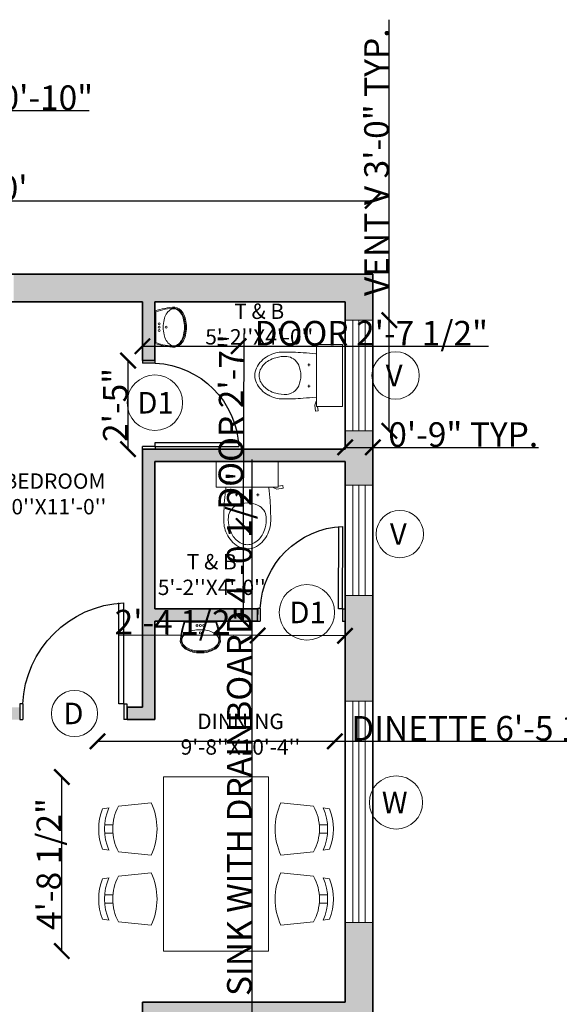
# Model space of a CAD drawing. Units: inches. Extents: x 2209 to 2954, y 1760 to 2265.
# Tile 4 of 7: x 2404 to 2580, y 1945 to 2265. Entities that reach past the tile are written whole.
import ezdxf

# ---------------------------------------------------------------- set-up
doc = ezdxf.new("R2010")
doc.units = ezdxf.units.IN
for name, color, linetype, lineweight in [('A-ANNO-DIMS', 2, 'Continuous', 18), ('A-ANNO-SYMB', 7, 'Continuous', 18), ('A-AREA-IDEN', 7, 'Continuous', 18), ('A-FLOR-FIXT', 9, 'Continuous', 18), ('A-FURN', 8, 'Continuous', 18), ('A-WALL-PATT', 30, 'Continuous', 13), ('DOOR', 240, 'Continuous', 25), ('WALL', 7, 'Continuous', 35), ('WINDOW', 190, 'Continuous', 18)]:
    doc.layers.add(name, color=color, linetype=linetype, lineweight=lineweight)
doc.styles.get("Standard").update_dxf_attribs({"font": 'arial.ttf'})
doc.dimstyles.get("Standard").update_dxf_attribs({"dimtxt": 8, "dimasz": 5, "dimexe": 0.18, "dimexo": 0.0625, "dimgap": 0.09, "dimtad": 1, "dimdec": 1, "dimzin": 0, "dimdsep": 46, "dimlunit": 4, "dimtxsty": 'Standard', "dimblk": 'ARCHTICK', "dimcen": 0.09, "dimse1": 1, "dimse2": 1, "dimadec": 0, "dimazin": 0, "dimtfac": 1, "dimtdec": 1, "dimtofl": 0, "dimtmove": 0, "dimatfit": 3, "dimfxl": 1, "dimtolj": 1, "dimtzin": 0, "dimarcsym": 0})

# ---------------------------------------------------------------- blocks, each defined once
blk = doc.blocks.new('table-23')
at = {"color": 0, "linetype": 'ByBlock'}
for p, q in [((-0.9, -1.4923), (-0.9, 0)), ((-0.9, 0), (0, 0)), ((0, -1.4923), (0, 0)), ((-1.0062, -0.2211), (-1.2862, -0.2511)), ((0.1062, -0.2211), (0.3862, -0.2511)), ((-1.3677, -0.2639), (-1.4237, -0.2726)), ((0.4677, -0.2639), (0.5237, -0.2726)), ((-1.4049, -0.4111), (-1.3347, -0.4111)), ((0.5049, -0.4111), (0.4347, -0.4111)), ((-1.4049, -0.4811), (-1.3347, -0.4811)), ((0.5049, -0.4811), (0.4347, -0.4811)), ((-1.3677, -0.6284), (-1.4237, -0.6197)), ((-1.0062, -0.6711), (-1.2862, -0.6411)), ((0.1062, -0.6711), (0.3862, -0.6411)), ((0.4677, -0.6284), (0.5237, -0.6197)), ((-1.0062, -0.8211), (-1.2862, -0.8511)), ((0.1062, -0.8211), (0.3862, -0.8511)), ((-1.3677, -0.8639), (-1.4237, -0.8726)), ((0.4677, -0.8639), (0.5237, -0.8726)), ((-1.4049, -1.0111), (-1.3347, -1.0111)), ((0.5049, -1.0111), (0.4347, -1.0111)), ((-1.4049, -1.0811), (-1.3347, -1.0811)), ((0.5049, -1.0811), (0.4347, -1.0811)), ((-1.3677, -1.2284), (-1.4237, -1.2197)), ((-1.0062, -1.2711), (-1.2862, -1.2411)), ((0.1062, -1.2711), (0.3862, -1.2411)), ((0.4677, -1.2284), (0.5237, -1.2197)), ((-0.9, -1.4923), (0, -1.4923))]:
    blk.add_line(p, q, dxfattribs=at)
for centre, radius, start, end in [((-0.931, -0.4461), 0.4053, 151.23721, 208.76279), ((-1.4875, -0.4461), 0.5312, 334.94238, 25.05762), ((0.5875, -0.4461), 0.5312, 154.94238, 205.05762), ((0.031, -0.4461), 0.4053, 331.23721, 28.76279), ((-0.9765, -0.4461), 0.4797, 158.78869, 201.21131), ((-0.9558, -0.4461), 0.4505, 156.13443, 203.86557), ((0.0558, -0.4461), 0.4505, 336.13443, 23.86557), ((0.0765, -0.4461), 0.4797, 338.78869, 21.21131), ((-1.4875, -1.0461), 0.5312, 334.94238, 25.05762), ((0.5875, -1.0461), 0.5312, 154.94238, 205.05762), ((-0.9765, -1.0461), 0.4797, 158.78869, 201.21131), ((-0.9558, -1.0461), 0.4505, 156.13443, 203.86557), ((-0.931, -1.0461), 0.4053, 151.23721, 208.76279), ((0.031, -1.0461), 0.4053, 331.23721, 28.76279), ((0.0558, -1.0461), 0.4505, 336.13443, 23.86557), ((0.0765, -1.0461), 0.4797, 338.78869, 21.21131)]:
    blk.add_arc(centre, radius, start, end, dxfattribs=at)
blk = doc.blocks.new('AP0B05')
for p, q in [((35, 100), (35, 880)), ((75, 100), (75, 878.9)), ((35, 100), (11, 100)), ((11, 100), (11, -20)), ((35, 100), (35, -20)), ((815, 100), (815, -20)), ((815, 100), (839, 100)), ((839, 100), (839, -20)), ((11, -20), (35, -20)), ((839, -20), (815, -20))]:
    blk.add_line(p, q)
blk.add_lwpolyline([(35, 100), (75, 100)])
blk.add_arc((-2.4, 62.6), 818.3, 2.62122, 87.37878)
blk = doc.blocks.new('toilet-1')
at = {"color": 0, "linetype": 'ByBlock'}
for p, q in [((-0.23, -0.02), (-0.23, -0.2116)), ((0.23, -0.02), (-0.23, -0.02)), ((0.23, -0.02), (0.23, -0.2116)), ((-0.23, -0.2116), (0.23, -0.2116)), ((0.1917, -0.2144), (0.2206, -0.225)), ((0.2206, -0.225), (0.266, -0.2187)), ((0.2633, -0.1997), (0.23, -0.2044)), ((0.266, -0.2187), (0.2633, -0.1997)), ((-0.0889, -0.2683), (-0.0697, -0.2683)), ((-0.0793, -0.2587), (-0.0793, -0.2778)), ((0.0889, -0.2683), (0.0698, -0.2683)), ((0.0794, -0.2587), (0.0794, -0.2778)), ((0, -0.6382), (0, -0.6382))]:
    blk.add_line(p, q, dxfattribs=at)
for centre, radius, start, end in [((3.5272, -0.6239), 3.7093, 173.69251, 175.15926), ((-3.527, -0.624), 3.7093, 4.84131, 6.31706), ((1.7368, -0.4519), 1.9109, 175.76982, 180.37578), ((-0.0312, -0.4465), 0.1114, 113.89968, 145.1485), ((0, -0.5169), 0.1884, 66.09393, 113.90607), ((0.0312, -0.4465), 0.1114, 34.8515, 66.10032), ((-1.7366, -0.4519), 1.9109, 359.62422, 4.23018), ((0.0981, -0.4497), 0.2389, 175.88621, 195.59308), ((-0.0408, -0.4398), 0.0996, 145.14967, 175.88096), ((0.0409, -0.4398), 0.0996, 4.11904, 34.85033), ((-0.098, -0.4497), 0.2389, 344.40692, 4.11379), ((0.0353, -0.463), 0.2093, 180.37466, 194.33753), ((-0.0351, -0.463), 0.2093, 345.6614, 359.62427), ((0.055, -0.458), 0.2297, 194.33532, 209.62204), ((0.0647, -0.4524), 0.2409, 209.62726, 224.54888), ((0.0961, -0.4503), 0.2369, 195.59686, 209.37705), ((0.0232, -0.4913), 0.1532, 209.38715, 226.54376), ((-0.0231, -0.4913), 0.1532, 313.45624, 330.61285), ((-0.0645, -0.4524), 0.2409, 315.45042, 330.37204), ((-0.096, -0.4503), 0.2369, 330.62295, 344.40314), ((-0.0548, -0.458), 0.2297, 330.37879, 345.66551), ((0.0178, -0.4986), 0.1751, 224.55199, 245.714), ((0.0152, -0.4997), 0.1416, 226.55015, 246.55272), ((0, -0.5347), 0.1034, 246.54933, 270.0042), ((0, -0.5347), 0.1034, 269.9958, 293.45067), ((-0.0151, -0.4997), 0.1416, 293.44728, 313.44985), ((-0.0176, -0.4986), 0.1751, 294.28649, 315.4485), ((0.0004, -0.538), 0.132, 245.58449, 269.87817), ((-0.0002, -0.538), 0.132, 270.12162, 294.4153)]:
    blk.add_arc(centre, radius, start, end, dxfattribs=at)
blk = doc.blocks.new('wash-3')
at = {"color": 0, "linetype": 'ByBlock'}
blk.add_line((0.23, -0.015), (-0.23, -0.015), dxfattribs=at)
for centre in [(-0.05, -0.066), (0, -0.066), (0.05, -0.066), (0, -0.172)]:
    blk.add_circle(centre, 0.0148, dxfattribs=at)
for centre, radius, start, end in [((0.69, -0.34), 0.991, 159.941, 177.839), ((0.69, -0.34), 0.976, 160.5399, 177.7326), ((-0.038, -0.45), 0.319, 103.3619, 119.8322), ((0, -0.61), 0.483, 90, 103.3619), ((0, -0.61), 0.483, 76.6381, 90), ((0.038, -0.45), 0.319, 60.1678, 76.6381), ((-0.69, -0.34), 0.976, 2.2674, 19.4601), ((-0.69, -0.34), 0.991, 2.161, 20.059), ((-0.183, -0.286), 0.095, 144.1588, 180), ((-0.183, -0.286), 0.095, 180, 215.8412), ((-0.096, -0.349), 0.203, 119.8322, 144.1588), ((0.096, -0.349), 0.203, 35.8412, 60.1678), ((0.183, -0.286), 0.095, 0, 35.8412), ((0.183, -0.286), 0.095, 324.1588, 0), ((-0.12, -0.265), 0.184, 191.7424, 233.4191), ((-0.12, -0.265), 0.169, 192.3358, 233.361), ((-0.096, -0.223), 0.203, 215.8412, 240.1678), ((-0.096, -0.223), 0.232, 234.7719, 240.1678), ((-0.096, -0.223), 0.217, 234.8176, 240.1678), ((-0.038, -0.122), 0.348, 240.1678, 256.6381), ((-0.038, -0.122), 0.333, 240.1678, 256.6381), ((-0.038, -0.122), 0.319, 240.1678, 256.6381), ((0, 0.038), 0.483, 256.6381, 270), ((0, 0.038), 0.483, 270, 283.3619), ((0.038, -0.122), 0.319, 283.3619, 299.8322), ((0.038, -0.122), 0.333, 283.3619, 299.8322), ((0.038, -0.122), 0.348, 283.3619, 299.8322), ((0.096, -0.223), 0.203, 299.8322, 324.1588), ((0.096, -0.223), 0.217, 299.8322, 305.1824), ((0.096, -0.223), 0.232, 299.8322, 305.2281), ((0.12, -0.265), 0.169, 306.639, 347.6642), ((0.12, -0.265), 0.184, 306.5809, 348.2576), ((0, 0.038), 0.513, 256.6381, 270), ((0, 0.038), 0.498, 256.6381, 270), ((0, 0.038), 0.498, 270, 283.3619), ((0, 0.038), 0.513, 270, 283.3619)]:
    blk.add_arc(centre, radius, start, end, dxfattribs=at)
blk = doc.blocks.new('_ArchTick')
at = {"color": 0, "linetype": 'ByBlock', "const_width": 0.15}
blk.add_lwpolyline([(-0.5, -0.5), (0.5, 0.5)], dxfattribs=at)
blk = doc.blocks.new('*D13')
at = {"layer": 'A-ANNO-DIMS', "color": 0, "lineweight": -2, "transparency": 16777216}
blk.add_line((2279.15, 2206.17), (2519.15, 2206.17), dxfattribs=at)
at = {"layer": 'Defpoints', "color": 0, "transparency": 16777216}
for p in [(2519.15, 2206.17), (2279.15, 2182.29), (2519.15, 2182.29)]:
    blk.add_point(p, dxfattribs=at)
at = {"layer": 'A-ANNO-DIMS', "color": 0, "lineweight": -2, "transparency": 16777216, "xscale": 5, "yscale": 5, "zscale": 5, "rotation": 180}
blk.add_blockref('_ArchTick', (2279.15, 2206.17), dxfattribs=at)
at = {"layer": 'A-ANNO-DIMS', "color": 0, "lineweight": -2, "transparency": 16777216, "xscale": 5, "yscale": 5, "zscale": 5}
blk.add_blockref('_ArchTick', (2519.15, 2206.17), dxfattribs=at)
at = {"layer": 'A-ANNO-DIMS', "color": 0, "transparency": 16777216, "insert": (2399.15, 2210.34), "char_height": 8, "attachment_point": 5}
blk.add_mtext("\\A1;20'", dxfattribs=at)
blk = doc.blocks.new('WIN-W-72IN')
for p, q in [((0, 6.5), (72, 6.5)), ((0, 4.5), (72, 4.5)), ((0, 2.5), (72, 2.5))]:
    blk.add_line(p, q)
blk.add_lwpolyline([(0, 9), (72, 9), (72, 0), (0, 0)], close=True)
blk = doc.blocks.new('VENT-V-36IN')
for p, q in [((2.5, 0), (2.5, 36)), ((4.5, 0), (4.5, 36)), ((6.5, 0), (6.5, 36))]:
    blk.add_line(p, q)
blk.add_lwpolyline([(0, 0), (0, 36), (9, 36), (9, 0)], close=True)
blk = doc.blocks.new('TAG-OPENING-W')
blk.add_circle((0, 0), 8.66)
blk.add_text('W', height=7).set_placement((-4.62, -3.5))
blk = doc.blocks.new('TAG-OPENING-V')
blk.add_circle((0, 0), 7.71)
blk.add_text('V', height=7).set_placement((-3.24, -3.5))
blk = doc.blocks.new('TAG-OPENING-D')
blk.add_circle((0, 0), 7.5)
blk.add_text('D', height=7).set_placement((-3.65, -3.5))
blk = doc.blocks.new('TAG-OPENING-D1')
blk.add_circle((0, 0), 9.03)
blk.add_text('D1', height=7).set_placement((-5.73, -3.51))
blk = doc.blocks.new('*D31')
at = {"layer": 'A-ANNO-DIMS', "color": 0, "lineweight": -2, "transparency": 16777216}
for p, q in [((2524.55, 2167.29), (2524.55, 2265.11)), ((2524.55, 2131.29), (2524.55, 2167.29))]:
    blk.add_line(p, q, dxfattribs=at)
at = {"layer": 'Defpoints', "color": 0, "transparency": 16777216}
for p in [(2519.15, 2167.29), (2524.55, 2167.29), (2519.15, 2131.29)]:
    blk.add_point(p, dxfattribs=at)
at = {"layer": 'A-ANNO-DIMS', "color": 0, "lineweight": -2, "transparency": 16777216, "xscale": 5, "yscale": 5, "zscale": 5}
for p, rotation in [((2524.55, 2167.29), 90), ((2524.55, 2131.29), 270)]:
    blk.add_blockref('_ArchTick', p, dxfattribs=dict(at, rotation=rotation))
at = {"layer": 'A-ANNO-DIMS', "color": 0, "transparency": 16777216, "insert": (2520.38, 2218.7), "char_height": 8, "attachment_point": 5, "rotation": 90}
blk.add_mtext('\\A1;VENT V 3\'-0" TYP.', dxfattribs=at)
blk = doc.blocks.new('*D32')
at = {"layer": 'A-ANNO-DIMS', "color": 0, "lineweight": -2, "transparency": 16777216}
for p, q in [((2510.15, 2125.89), (2519.15, 2125.89)), ((2519.15, 2125.89), (2573.1, 2125.89))]:
    blk.add_line(p, q, dxfattribs=at)
at = {"layer": 'Defpoints', "color": 0, "transparency": 16777216}
for p in [(2510.15, 2131.29), (2519.15, 2131.29), (2519.15, 2125.89)]:
    blk.add_point(p, dxfattribs=at)
at = {"layer": 'A-ANNO-DIMS', "color": 0, "lineweight": -2, "transparency": 16777216, "xscale": 5, "yscale": 5, "zscale": 5, "rotation": 180}
blk.add_blockref('_ArchTick', (2510.15, 2125.89), dxfattribs=at)
at = {"layer": 'A-ANNO-DIMS', "color": 0, "lineweight": -2, "transparency": 16777216, "xscale": 5, "yscale": 5, "zscale": 5}
blk.add_blockref('_ArchTick', (2519.15, 2125.89), dxfattribs=at)
at = {"layer": 'A-ANNO-DIMS', "color": 0, "transparency": 16777216, "insert": (2548.63, 2130.06), "char_height": 8, "attachment_point": 5}
blk.add_mtext('\\A1;0\'-9" TYP.', dxfattribs=at)
blk = doc.blocks.new('*D43')
at = {"layer": 'A-ANNO-DIMS', "color": 0, "lineweight": -2, "transparency": 16777216}
for p, q in [((2444.15, 2158.82), (2475.5, 2158.82)), ((2475.5, 2158.82), (2556.82, 2158.82))]:
    blk.add_line(p, q, dxfattribs=at)
at = {"layer": 'Defpoints', "color": 0, "transparency": 16777216}
for p in [(2475.5, 2158.82), (2444.15, 2154.12), (2475.5, 2154.12)]:
    blk.add_point(p, dxfattribs=at)
at = {"layer": 'A-ANNO-DIMS', "color": 0, "lineweight": -2, "transparency": 16777216, "xscale": 5, "yscale": 5, "zscale": 5, "rotation": 180}
blk.add_blockref('_ArchTick', (2444.15, 2158.82), dxfattribs=at)
at = {"layer": 'A-ANNO-DIMS', "color": 0, "lineweight": -2, "transparency": 16777216, "xscale": 5, "yscale": 5, "zscale": 5}
blk.add_blockref('_ArchTick', (2475.5, 2158.82), dxfattribs=at)
at = {"layer": 'A-ANNO-DIMS', "color": 0, "transparency": 16777216, "insert": (2518.66, 2163.05), "char_height": 8, "attachment_point": 5}
blk.add_mtext('\\A1;DOOR 2\'-7 1/2"', dxfattribs=at)
blk = doc.blocks.new('*D44')
at = {"layer": 'A-ANNO-DIMS', "color": 0, "lineweight": -2, "transparency": 16777216}
blk.add_line((2439.45, 2125.29), (2439.45, 2154.12), dxfattribs=at)
at = {"layer": 'Defpoints', "color": 0, "transparency": 16777216}
for p in [(2439.45, 2154.12), (2444.15, 2154.12), (2444.15, 2125.29)]:
    blk.add_point(p, dxfattribs=at)
at = {"layer": 'A-ANNO-DIMS', "color": 0, "lineweight": -2, "transparency": 16777216, "xscale": 5, "yscale": 5, "zscale": 5}
for p, rotation in [((2439.45, 2154.12), 90), ((2439.45, 2125.29), 270)]:
    blk.add_blockref('_ArchTick', p, dxfattribs=dict(at, rotation=rotation))
at = {"layer": 'A-ANNO-DIMS', "color": 0, "transparency": 16777216, "insert": (2435.28, 2139.7), "char_height": 8, "attachment_point": 5, "rotation": 90}
blk.add_mtext('\\A1;2\'-5"', dxfattribs=at)
blk = doc.blocks.new('*D45')
at = {"layer": 'A-ANNO-DIMS', "color": 0, "lineweight": -2, "transparency": 16777216}
for p, q in [((2477.11, 2100.28), (2477.31, 2162.96)), ((2477.01, 2069.3), (2477.11, 2100.28))]:
    blk.add_line(p, q, dxfattribs=at)
at = {"layer": 'Defpoints', "color": 0, "transparency": 16777216}
for p in [(2477.11, 2100.28), (2481.76, 2100.26), (2481.65, 2069.29)]:
    blk.add_point(p, dxfattribs=at)
at = {"layer": 'A-ANNO-DIMS', "color": 0, "lineweight": -2, "transparency": 16777216, "xscale": 5, "yscale": 5, "zscale": 5}
for p, rotation in [((2477.11, 2100.28), 89.81328114841703), ((2477.01, 2069.3), 269.8132811484171)]:
    blk.add_blockref('_ArchTick', p, dxfattribs=dict(at, rotation=rotation))
at = {"layer": 'A-ANNO-DIMS', "color": 0, "transparency": 16777216, "insert": (2472.99, 2134.13), "char_height": 8, "attachment_point": 5, "rotation": 89.8133}
blk.add_mtext('\\A1;DOOR 2\'-7"', dxfattribs=at)
blk = doc.blocks.new('*D46')
at = {"layer": 'A-ANNO-DIMS', "color": 0, "lineweight": -2, "transparency": 16777216}
for p, q in [((2481.64, 2064.64), (2436.42, 2064.79)), ((2510.14, 2064.55), (2481.64, 2064.64))]:
    blk.add_line(p, q, dxfattribs=at)
at = {"layer": 'Defpoints', "color": 0, "transparency": 16777216}
for p in [(2481.65, 2069.29), (2510.15, 2069.19), (2481.64, 2064.64)]:
    blk.add_point(p, dxfattribs=at)
at = {"layer": 'A-ANNO-DIMS', "color": 0, "lineweight": -2, "transparency": 16777216, "xscale": 5, "yscale": 5, "zscale": 5}
for p, rotation in [((2481.64, 2064.64), 179.8132811484169), ((2510.14, 2064.55), 359.8132811484169)]:
    blk.add_blockref('_ArchTick', p, dxfattribs=dict(at, rotation=rotation))
at = {"layer": 'A-ANNO-DIMS', "color": 0, "transparency": 16777216, "insert": (2456.54, 2068.95), "char_height": 8, "attachment_point": 5, "rotation": 359.8133}
blk.add_mtext('\\A1;2\'-4 1/2"', dxfattribs=at)
blk = doc.blocks.new('*D53')
at = {"layer": 'A-ANNO-DIMS', "color": 0, "lineweight": -2, "transparency": 16777216}
blk.add_line((2385.75, 2056.56), (2385.75, 2158.01), dxfattribs=at)
at = {"layer": 'Defpoints', "color": 0, "transparency": 16777216}
for p in [(2370.53, 2158.01), (2385.75, 2158.01), (2370.53, 2056.56)]:
    blk.add_point(p, dxfattribs=at)
at = {"layer": 'A-ANNO-DIMS', "color": 0, "lineweight": -2, "transparency": 16777216, "xscale": 5, "yscale": 5, "zscale": 5}
for p, rotation in [((2385.75, 2158.01), 90), ((2385.75, 2056.56), 270)]:
    blk.add_blockref('_ArchTick', p, dxfattribs=dict(at, rotation=rotation))
at = {"layer": 'A-ANNO-DIMS', "color": 0, "transparency": 16777216, "insert": (2381.53, 2107.29), "char_height": 8, "attachment_point": 5, "rotation": 90}
blk.add_mtext('\\A1;BED 8\'-5 1/2" TYP.', dxfattribs=at)
blk = doc.blocks.new('*D61')
at = {"layer": 'A-ANNO-DIMS', "color": 0, "lineweight": -2, "transparency": 16777216}
for p, q in [((2429.48, 2030.19), (2506.77, 2030.19)), ((2506.77, 2030.19), (2602.37, 2030.19))]:
    blk.add_line(p, q, dxfattribs=at)
at = {"layer": 'Defpoints', "color": 0, "transparency": 16777216}
for p in [(2506.77, 2030.19), (2429.48, 2018.6), (2506.77, 2018.6)]:
    blk.add_point(p, dxfattribs=at)
at = {"layer": 'A-ANNO-DIMS', "color": 0, "lineweight": -2, "transparency": 16777216, "xscale": 5, "yscale": 5, "zscale": 5, "rotation": 180}
blk.add_blockref('_ArchTick', (2429.48, 2030.19), dxfattribs=at)
at = {"layer": 'A-ANNO-DIMS', "color": 0, "lineweight": -2, "transparency": 16777216, "xscale": 5, "yscale": 5, "zscale": 5}
blk.add_blockref('_ArchTick', (2506.77, 2030.19), dxfattribs=at)
at = {"layer": 'A-ANNO-DIMS', "color": 0, "transparency": 16777216, "insert": (2557.07, 2034.42), "char_height": 8, "attachment_point": 5}
blk.add_mtext('\\A1;DINETTE 6\'-5 1/2"', dxfattribs=at)
blk = doc.blocks.new('*D62')
at = {"layer": 'A-ANNO-DIMS', "color": 0, "lineweight": -2, "transparency": 16777216}
blk.add_line((2417.88, 1961.89), (2417.88, 2018.6), dxfattribs=at)
at = {"layer": 'Defpoints', "color": 0, "transparency": 16777216}
for p in [(2417.88, 2018.6), (2429.48, 2018.6), (2429.48, 1961.89)]:
    blk.add_point(p, dxfattribs=at)
at = {"layer": 'A-ANNO-DIMS', "color": 0, "lineweight": -2, "transparency": 16777216, "xscale": 5, "yscale": 5, "zscale": 5}
for p, rotation in [((2417.88, 2018.6), 90), ((2417.88, 1961.89), 270)]:
    blk.add_blockref('_ArchTick', p, dxfattribs=dict(at, rotation=rotation))
at = {"layer": 'A-ANNO-DIMS', "color": 0, "transparency": 16777216, "insert": (2413.65, 1990.24), "char_height": 8, "attachment_point": 5, "rotation": 90}
blk.add_mtext('\\A1;4\'-8 1/2"', dxfattribs=at)
blk = doc.blocks.new('*D65')
at = {"layer": 'A-ANNO-DIMS', "color": 0, "lineweight": -2, "transparency": 16777216}
for p, q in [((2479.92, 1938.37), (2479.92, 2121.89)), ((2479.92, 1889.91), (2479.92, 1938.37))]:
    blk.add_line(p, q, dxfattribs=at)
at = {"layer": 'Defpoints', "color": 0, "transparency": 16777216}
for p in [(2479.92, 1938.37), (2487.19, 1938.37), (2487.19, 1889.91)]:
    blk.add_point(p, dxfattribs=at)
at = {"layer": 'A-ANNO-DIMS', "color": 0, "lineweight": -2, "transparency": 16777216, "xscale": 5, "yscale": 5, "zscale": 5}
for p, rotation in [((2479.92, 1938.37), 90), ((2479.92, 1889.91), 270)]:
    blk.add_blockref('_ArchTick', p, dxfattribs=dict(at, rotation=rotation))
at = {"layer": 'A-ANNO-DIMS', "color": 0, "transparency": 16777216, "insert": (2475.69, 2032.63), "char_height": 8, "attachment_point": 5, "rotation": 90}
blk.add_mtext('\\A1;SINK WITH DRAINBOARD 4\'-0 1/2"', dxfattribs=at)
blk = doc.blocks.new('*D75')
at = {"layer": 'A-ANNO-DIMS', "color": 0, "lineweight": -2, "transparency": 16777216}
blk.add_line((2920.04, 1922.29), (2920.04, 1971.25), dxfattribs=at)
at = {"layer": 'Defpoints', "color": 0, "transparency": 16777216}
for p in [(2519.15, 1971.25), (2920.04, 1971.25), (2519.15, 1922.29)]:
    blk.add_point(p, dxfattribs=at)
at = {"layer": 'A-ANNO-DIMS', "color": 0, "lineweight": -2, "transparency": 16777216, "xscale": 5, "yscale": 5, "zscale": 5}
for p, rotation in [((2920.04, 1971.25), 90), ((2920.04, 1922.29), 270)]:
    blk.add_blockref('_ArchTick', p, dxfattribs=dict(at, rotation=rotation))
at = {"layer": 'A-ANNO-DIMS', "color": 0, "transparency": 16777216, "insert": (2915.94, 1946.77), "char_height": 8, "attachment_point": 5, "rotation": 90}
blk.add_mtext('\\A1;4\'-1"', dxfattribs=at)
blk = doc.blocks.new('*D76')
at = {"layer": 'A-ANNO-DIMS', "color": 0, "lineweight": -2, "transparency": 16777216}
for p, q in [((2920.04, 2077.63), (2920.04, 2129.07)), ((2920.04, 2043.25), (2920.04, 2077.63))]:
    blk.add_line(p, q, dxfattribs=at)
at = {"layer": 'Defpoints', "color": 0, "transparency": 16777216}
for p in [(2519.15, 2077.63), (2920.04, 2077.63), (2519.15, 2043.25)]:
    blk.add_point(p, dxfattribs=at)
at = {"layer": 'A-ANNO-DIMS', "color": 0, "lineweight": -2, "transparency": 16777216, "xscale": 5, "yscale": 5, "zscale": 5}
for p, rotation in [((2920.04, 2077.63), 90), ((2920.04, 2043.25), 270)]:
    blk.add_blockref('_ArchTick', p, dxfattribs=dict(at, rotation=rotation))
at = {"layer": 'A-ANNO-DIMS', "color": 0, "transparency": 16777216, "insert": (2915.82, 2105.85), "char_height": 8, "attachment_point": 5, "rotation": 90}
blk.add_mtext('\\A1;2\'-10 1/2"', dxfattribs=at)
blk = doc.blocks.new('*D77')
at = {"layer": 'A-ANNO-DIMS', "color": 0, "lineweight": -2, "transparency": 16777216}
for p, q in [((2920.04, 2131.29), (2920.04, 2175.62)), ((2920.04, 2113.63), (2920.04, 2131.29))]:
    blk.add_line(p, q, dxfattribs=at)
at = {"layer": 'Defpoints', "color": 0, "transparency": 16777216}
for p in [(2519.15, 2131.29), (2920.04, 2131.29), (2519.15, 2113.63)]:
    blk.add_point(p, dxfattribs=at)
at = {"layer": 'A-ANNO-DIMS', "color": 0, "lineweight": -2, "transparency": 16777216, "xscale": 5, "yscale": 5, "zscale": 5}
for p, rotation in [((2920.04, 2131.29), 90), ((2920.04, 2113.63), 270)]:
    blk.add_blockref('_ArchTick', p, dxfattribs=dict(at, rotation=rotation))
at = {"layer": 'A-ANNO-DIMS', "color": 0, "transparency": 16777216, "insert": (2915.82, 2155.95), "char_height": 8, "attachment_point": 5, "rotation": 90}
blk.add_mtext('\\A1;1\'-5 1/2"', dxfattribs=at)
blk = doc.blocks.new('*D79')
at = {"layer": 'A-ANNO-DIMS', "color": 0, "lineweight": -2, "transparency": 16777216}
for p, q in [((2384.15, 2235.55), (2394.15, 2235.55)), ((2394.15, 2235.55), (2426.82, 2235.55))]:
    blk.add_line(p, q, dxfattribs=at)
at = {"layer": 'Defpoints', "color": 0, "transparency": 16777216}
for p in [(2394.15, 2235.55), (2384.15, 1981.29), (2394.15, 1981.29)]:
    blk.add_point(p, dxfattribs=at)
at = {"layer": 'A-ANNO-DIMS', "color": 0, "lineweight": -2, "transparency": 16777216, "xscale": 5, "yscale": 5, "zscale": 5, "rotation": 180}
blk.add_blockref('_ArchTick', (2384.15, 2235.55), dxfattribs=at)
at = {"layer": 'A-ANNO-DIMS', "color": 0, "lineweight": -2, "transparency": 16777216, "xscale": 5, "yscale": 5, "zscale": 5}
blk.add_blockref('_ArchTick', (2394.15, 2235.55), dxfattribs=at)
at = {"layer": 'A-ANNO-DIMS', "color": 0, "transparency": 16777216, "insert": (2412.99, 2239.72), "char_height": 8, "attachment_point": 5}
blk.add_mtext('\\A1;0\'-10"', dxfattribs=at)
blk = doc.blocks.new('*D87')
at = {"layer": 'A-ANNO-DIMS', "color": 0, "lineweight": -2, "transparency": 16777216}
blk.add_line((2224.78, 2146.27), (2224.78, 2182.29), dxfattribs=at)
at = {"layer": 'Defpoints', "color": 0, "transparency": 16777216}
for p in [(2224.78, 2182.29), (2629.22, 2182.29), (2629.22, 2146.27)]:
    blk.add_point(p, dxfattribs=at)
at = {"layer": 'A-ANNO-DIMS', "color": 0, "lineweight": -2, "transparency": 16777216, "xscale": 5, "yscale": 5, "zscale": 5}
for p, rotation in [((2224.78, 2182.29), 90), ((2224.78, 2146.27), 270)]:
    blk.add_blockref('_ArchTick', p, dxfattribs=dict(at, rotation=rotation))
at = {"layer": 'A-ANNO-DIMS', "color": 0, "transparency": 16777216, "insert": (2220.6, 2164.28), "char_height": 8, "attachment_point": 5, "rotation": 90}
blk.add_mtext('\\A1;3\'-0"', dxfattribs=at)
blk = doc.blocks.new('*D88')
at = {"layer": 'A-ANNO-DIMS', "color": 0, "lineweight": -2, "transparency": 16777216}
blk.add_line((2224.78, 1919.53), (2224.78, 1973.14), dxfattribs=at)
at = {"layer": 'Defpoints', "color": 0, "transparency": 16777216}
for p in [(2224.78, 1973.14), (2629.22, 1973.14), (2629.22, 1919.53)]:
    blk.add_point(p, dxfattribs=at)
at = {"layer": 'A-ANNO-DIMS', "color": 0, "lineweight": -2, "transparency": 16777216, "xscale": 5, "yscale": 5, "zscale": 5}
for p, rotation in [((2224.78, 1973.14), 90), ((2224.78, 1919.53), 270)]:
    blk.add_blockref('_ArchTick', p, dxfattribs=dict(at, rotation=rotation))
at = {"layer": 'A-ANNO-DIMS', "color": 0, "transparency": 16777216, "insert": (2220.55, 1946.34), "char_height": 8, "attachment_point": 5, "rotation": 90}
blk.add_mtext('\\A1;4\'-5 1/2"', dxfattribs=at)
blk = doc.blocks.new('*D89')
at = {"layer": 'A-ANNO-DIMS', "color": 0, "lineweight": -2, "transparency": 16777216}
blk.add_line((2224.78, 2009.14), (2224.78, 2074.27), dxfattribs=at)
at = {"layer": 'Defpoints', "color": 0, "transparency": 16777216}
for p in [(2224.78, 2074.27), (2629.22, 2074.27), (2629.22, 2009.14)]:
    blk.add_point(p, dxfattribs=at)
at = {"layer": 'A-ANNO-DIMS', "color": 0, "lineweight": -2, "transparency": 16777216, "xscale": 5, "yscale": 5, "zscale": 5}
for p, rotation in [((2224.78, 2074.27), 90), ((2224.78, 2009.14), 270)]:
    blk.add_blockref('_ArchTick', p, dxfattribs=dict(at, rotation=rotation))
at = {"layer": 'A-ANNO-DIMS', "color": 0, "transparency": 16777216, "insert": (2220.62, 2041.7), "char_height": 8, "attachment_point": 5, "rotation": 90}
blk.add_mtext('\\A1;5\'-5"', dxfattribs=at)
blk = doc.blocks.new('*D93')
at = {"layer": 'A-ANNO-DIMS', "color": 0, "lineweight": -2, "transparency": 16777216}
for p, q in [((2224.78, 2107.29), (2224.78, 2133.73)), ((2224.78, 2103.29), (2224.78, 2107.29))]:
    blk.add_line(p, q, dxfattribs=at)
at = {"layer": 'Defpoints', "color": 0, "transparency": 16777216}
for p in [(2224.78, 2107.29), (2798.22, 2107.29), (2798.22, 2103.29)]:
    blk.add_point(p, dxfattribs=at)
at = {"layer": 'A-ANNO-DIMS', "color": 0, "lineweight": -2, "transparency": 16777216, "xscale": 5, "yscale": 5, "zscale": 5}
for p, rotation in [((2224.78, 2107.29), 90), ((2224.78, 2103.29), 270)]:
    blk.add_blockref('_ArchTick', p, dxfattribs=dict(at, rotation=rotation))
at = {"layer": 'A-ANNO-DIMS', "color": 0, "transparency": 16777216, "insert": (2220.61, 2123.01), "char_height": 8, "attachment_point": 5, "rotation": 90}
blk.add_mtext('\\A1;0\'-4"', dxfattribs=at)

msp = doc.modelspace()

# ---------------------------------------------------------------- hatches: boundary and pattern name
at = {"layer": 'A-WALL-PATT', "transparency": 33554585}
h = msp.add_hatch(color=256, dxfattribs=at)
h.dxf.hatch_style = 1
h.paths.add_polyline_path([(2519.15, 2182.29), (2402.15, 2182.29), (2402.15, 2173.29), (2444.15, 2173.29), (2444.15, 2154.12), (2448.15, 2154.12), (2448.15, 2173.29), (2510.15, 2173.29), (2510.15, 2167.29), (2519.15, 2167.29)])
h.paths.add_polyline_path([(2330.15, 2182.29), (2279.15, 2182.29), (2279.15, 2145.83), (2288.15, 2145.83), (2288.15, 2158.01), (2288.15, 2173.29), (2330.15, 2173.29)])
h.paths.add_polyline_path([(2288.15, 2073.83), (2279.15, 2073.83), (2279.15, 2009.29), (2288.15, 2009.29), (2288.15, 2037.29), (2404.15, 2037.29), (2404.15, 2041.29), (2288.15, 2041.29)])
h.paths.add_polyline_path([(2519.15, 2131.29), (2510.15, 2131.29), (2510.15, 2125.29), (2444.15, 2125.29), (2444.15, 2041.29), (2439.11, 2041.29), (2439.11, 2037.29), (2448.15, 2037.29), (2448.15, 2069.29), (2481.65, 2069.29), (2481.65, 2073.29), (2448.15, 2073.29), (2448.15, 2121.29), (2468.19, 2121.29), (2468.19, 2121.32), (2488.37, 2121.32), (2510.15, 2121.29), (2510.15, 2113.63), (2519.15, 2113.63)])
h.paths.add_polyline_path([(2519.15, 2077.63), (2510.15, 2077.63), (2510.15, 2073.32), (2510.17, 2073.32), (2510.15, 2069.19), (2510.15, 2043.25), (2519.15, 2043.25)], flags=17)
h.paths.add_polyline_path([(2519.15, 1971.25), (2510.15, 1971.25), (2510.15, 1945.29), (2444.15, 1945.29), (2444.15, 1937.21), (2448.15, 1937.21), (2448.15, 1941.29), (2510.15, 1941.29), (2510.15, 1922.29), (2519.15, 1922.29)])
h.paths.add_polyline_path([(2288.15, 1941.29), (2394.15, 1941.29), (2394.15, 1945.29), (2288.15, 1945.29), (2288.15, 1973.29), (2279.15, 1973.29), (2279.15, 1919.97), (2288.15, 1919.97)])
h.paths.add_polyline_path([(2300.65, 1831.29), (2288.15, 1831.29), (2288.15, 1847.97), (2279.15, 1847.97), (2279.15, 1822.29), (2300.65, 1822.29)])
h.paths.add_polyline_path([(2394.15, 1825.29), (2394.15, 1831.29), (2372.65, 1831.29), (2372.65, 1822.29), (2394.15, 1822.29)])
h.paths.add_polyline_path([(2449.17, 1831.29), (2448.15, 1831.29), (2448.15, 1899.32), (2444.15, 1899.32), (2444.15, 1831.29), (2439.18, 1831.29), (2439.18, 1822.29), (2449.17, 1822.29)])
h.paths.add_polyline_path([(2519.15, 1850.29), (2510.15, 1850.29), (2510.15, 1831.29), (2509.17, 1831.29), (2509.17, 1822.29), (2519.15, 1822.29)])
h.paths.add_polyline_path([(2638.22, 1941.29), (2744.22, 1941.29), (2744.22, 1945.29), (2638.22, 1945.29), (2638.22, 1973.14), (2629.22, 1973.14), (2629.22, 1919.53), (2638.22, 1919.53)])
h.paths.add_polyline_path([(2638.22, 1847.53), (2629.22, 1847.53), (2629.22, 1822.29), (2650.72, 1822.29), (2650.72, 1831.29), (2638.22, 1831.29)])
h.paths.add_polyline_path([(2638.22, 2037.29), (2754.22, 2037.29), (2754.22, 2041.29), (2638.22, 2041.29), (2638.22, 2074.27), (2629.22, 2074.27), (2629.22, 2009.14), (2638.22, 2009.14)])
h.paths.add_polyline_path([(2803.22, 1936.29), (2812.78, 1936.29), (2812.78, 1945.29), (2791.22, 1945.29), (2791.22, 1936.29), (2794.22, 1936.29), (2794.22, 1831.29), (2722.72, 1831.29), (2722.72, 1822.29), (2803.22, 1822.29)])
h.paths.add_polyline_path([(2869.22, 1955.43), (2860.22, 1955.43), (2860.22, 1945.29), (2853.36, 1945.29), (2853.36, 1936.29), (2869.22, 1936.29)])
h.paths.add_polyline_path([(2680.22, 2182.29), (2629.22, 2182.29), (2629.22, 2146.27), (2638.22, 2146.27), (2638.22, 2173.29), (2680.22, 2173.29)])
h.paths.add_polyline_path([(2869.22, 2182.29), (2752.22, 2182.29), (2752.22, 2173.29), (2794.22, 2173.29), (2794.22, 2142.92), (2798.22, 2142.92), (2798.22, 2173.29), (2860.22, 2173.29), (2860.22, 2158.46), (2869.22, 2158.46)])
h.paths.add_polyline_path([(2869.22, 2122.46), (2860.22, 2122.46), (2860.22, 2090.29), (2869.22, 2090.29)])

# ---------------------------------------------------------------- linework, layer by layer
at = {"layer": 'WALL'}
for p, q in [((2279.15, 2182.29), (2519.15, 2182.29)), ((2519.15, 2182.29), (2519.15, 1822.29)), ((2288.15, 2173.29), (2444.15, 2173.29)), ((2444.15, 2173.29), (2444.15, 2154.12)), ((2448.15, 2173.29), (2448.15, 2154.12)), ((2448.15, 2173.29), (2510.15, 2173.29)), ((2510.15, 2173.29), (2510.15, 2125.29)), ((2444.15, 2154.12), (2448.15, 2154.12)), ((2444.15, 2125.29), (2510.15, 2125.29)), ((2444.15, 2125.29), (2444.15, 2041.29)), ((2448.15, 2121.29), (2510.15, 2121.29)), ((2448.15, 2121.29), (2448.15, 2073.29)), ((2510.15, 2121.29), (2510.15, 1945.29)), ((2448.15, 2073.29), (2481.65, 2073.29)), ((2481.65, 2069.29), (2481.65, 2073.29)), ((2448.15, 2069.29), (2481.65, 2069.29)), ((2448.15, 2069.29), (2448.15, 2037.29)), ((2439.11, 2041.29), (2439.11, 2037.29)), ((2439.11, 2041.29), (2444.15, 2041.29)), ((2439.11, 2037.29), (2448.15, 2037.29)), ((2444.15, 1945.29), (2444.15, 1937.21)), ((2444.15, 1945.29), (2510.15, 1945.29))]:
    msp.add_line(p, q, dxfattribs=at)

# ---------------------------------------------------------------- block references
at = {"layer": 'A-ANNO-SYMB'}
for name, p in [('TAG-OPENING-V', (2526.61, 2149.29)), ('TAG-OPENING-D1', (2448.19, 2140.42)), ('TAG-OPENING-V', (2527.98, 2097.67)), ('TAG-OPENING-D1', (2497.71, 2072.16)), ('TAG-OPENING-D', (2422.02, 2039.26)), ('TAG-OPENING-W', (2526.74, 2010.28))]:
    msp.add_blockref(name, p, dxfattribs=at)
at = {"layer": 'A-FLOR-FIXT'}
for name, p, xscale, yscale, zscale, rotation in [('wash-3', (2448.15, 2164.99), 21.75271524526245, 21.75271524526245, 21.75271524526245, 90), ('toilet-1', (2510.15, 2149.29), 43.86874267633562, 43.86874267633562, 43.86874267633562, 270)]:
    msp.add_blockref(name, p, dxfattribs=dict(at, xscale=xscale, yscale=yscale, zscale=zscale, rotation=rotation))
for name, p, xscale, yscale, zscale in [('toilet-1', (2478.28, 2122.2), 43.86874267633562, 43.86874267633562, 43.86874267633562), ('wash-3', (2463, 2069.29), 21.75271524526245, 21.75271524526245, 21.75271524526245)]:
    msp.add_blockref(name, p, dxfattribs=dict(at, xscale=xscale, yscale=yscale, zscale=zscale))
at = {"layer": 'A-FURN', "xscale": 37.99911430727016, "yscale": 37.99911430727016, "zscale": 37.99911430727016}
msp.add_blockref('table-23', (2485.22, 2018.6), dxfattribs=at)
at = {"layer": 'DOOR'}
for p, xscale, yscale, zscale, rotation in [((2444.85, 2124.9), -0.0348278393389822, 0.0348278393389822, 0.0348278393389822, 270), ((2510.54, 2069.88), -0.0344204726303782, 0.0344204726303782, 0.0344204726303782, 359.8132811484169)]:
    msp.add_blockref('AP0B05', p, dxfattribs=dict(at, xscale=xscale, yscale=yscale, zscale=zscale, rotation=rotation))
at = {"layer": 'DOOR', "xscale": -0.0422149343000146, "yscale": 0.0422149343000146, "zscale": 0.0422149343000146}
msp.add_blockref('AP0B05', (2439.57, 2038.13), dxfattribs=at)
at = {"layer": 'WINDOW'}
for p in [(2510.15, 2131.29), (2510.15, 2077.63)]:
    msp.add_blockref('VENT-V-36IN', p, dxfattribs=at)
at = {"layer": 'WINDOW', "rotation": 90.00000000000033}
msp.add_blockref('WIN-W-72IN', (2519.15, 1971.25), dxfattribs=at)

# ---------------------------------------------------------------- texts
at = {"layer": 'A-AREA-IDEN', "char_height": 5, "attachment_point": 1}
for s, insert in [("\\pxqc;T & B\\P5'-2''X4'-0''", (2459.61, 2172.7)), ("\\pxqc;M. BEDROOM\\P13'-0''X11'-0''", (2388.44, 2117.41)), ("\\pxqc;T & B\\P5'-2''X4'-0''", (2444.15, 2091.15)), ("\\pxqc;DINNING\\P9'-8''X10'-4''", (2453.5, 2039.18))]:
    msp.add_mtext_dynamic_manual_height_columns(s, width=45.1409, gutter_width=12.5, heights=[0], dxfattribs=dict(at, insert=insert))

# ---------------------------------------------------------------- dimensions: what is measured, and where the dimension line sits
at = {"layer": 'A-ANNO-DIMS'}
for base, p1, p2, angle, text, picture, middle in [((2524.55, 2167.29), (2519.15, 2131.29), (2519.15, 2167.29), 90, 'VENT V <> TYP.', '*D31', (2520.38, 2218.7)), ((2385.7523, 2158.0135), (2370.5338, 2056.5568), (2370.5338, 2158.0135), 90, 'BED <> TYP.', '*D53', (2381.5259, 2107.2851)), ((2477.11, 2100.28), (2481.65, 2069.29), (2481.76, 2100.26), 89.8133, 'DOOR <>', '*D45', (2472.99, 2134.13)), ((2479.92, 1938.37), (2487.19, 1889.91), (2487.19, 1938.37), 90, 'SINK WITH DRAINBOARD <>', '*D65', (2475.69, 2032.63))]:
    dim = msp.add_linear_dim(base=base, p1=p1, p2=p2, angle=angle, text=text, dimstyle='Standard', override={"dimdec": 1, "dimlfac": 1, "dimrnd": 0, "dimzin": 1, "dimdsep": 46, "dimlunit": 4, "dimfrac": 2}, dxfattribs=at)
    dim.commit()
    dim.dimension.update_dxf_attribs({"geometry": picture, "text_midpoint": middle})
for base, p1, p2, override, picture, middle in [((2394.15, 2235.55), (2384.15, 1981.29), (2394.15, 1981.29), {"dimdec": 1, "dimlfac": 1, "dimrnd": 0, "dimzin": 1, "dimdsep": 46, "dimlunit": 4, "dimfrac": 2}, '*D79', (2412.99, 2239.72)), ((2519.15, 2206.17), (2279.15, 2182.29), (2519.15, 2182.29), {"dimclrd": 0, "dimclre": 0, "dimclrt": 0}, '*D13', (2399.15, 2210.34))]:
    dim = msp.add_linear_dim(base=base, p1=p1, p2=p2, dimstyle='Standard', override=override, dxfattribs=at)
    dim.commit()
    dim.dimension.update_dxf_attribs({"geometry": picture, "text_midpoint": middle})
for base, p1, p2, angle, picture, middle in [((2224.78, 2182.29), (2629.22, 2146.27), (2629.22, 2182.29), 90, '*D87', (2220.6, 2164.28)), ((2920.04, 2131.29), (2519.15, 2113.63), (2519.15, 2131.29), 90, '*D77', (2915.82, 2155.95)), ((2439.45, 2154.12), (2444.15, 2125.29), (2444.15, 2154.12), 90, '*D44', (2435.28, 2139.7)), ((2224.78, 2107.29), (2798.22, 2103.29), (2798.22, 2107.29), 90, '*D93', (2220.61, 2123.01)), ((2920.04, 2077.63), (2519.15, 2043.25), (2519.15, 2077.63), 90, '*D76', (2915.82, 2105.85)), ((2481.64, 2064.64), (2510.15, 2069.19), (2481.65, 2069.29), 179.8133, '*D46', (2456.54, 2068.95)), ((2224.78, 2074.27), (2629.22, 2009.14), (2629.22, 2074.27), 90, '*D89', (2220.62, 2041.7)), ((2417.88, 2018.6), (2429.48, 1961.89), (2429.48, 2018.6), 90, '*D62', (2413.65, 1990.24)), ((2224.78, 1973.14), (2629.22, 1919.53), (2629.22, 1973.14), 90, '*D88', (2220.55, 1946.34)), ((2920.04, 1971.25), (2519.15, 1922.29), (2519.15, 1971.25), 90, '*D75', (2915.94, 1946.77))]:
    dim = msp.add_linear_dim(base=base, p1=p1, p2=p2, angle=angle, dimstyle='Standard', override={"dimdec": 1, "dimlfac": 1, "dimrnd": 0, "dimzin": 1, "dimdsep": 46, "dimlunit": 4, "dimfrac": 2}, dxfattribs=at)
    dim.commit()
    dim.dimension.update_dxf_attribs({"geometry": picture, "text_midpoint": middle})
for base, p1, p2, text, picture, middle in [((2475.4995, 2158.8244), (2444.1544, 2154.1226), (2475.4995, 2154.1226), 'DOOR <>', '*D43', (2518.6604, 2163.0535)), ((2519.15, 2125.89), (2510.15, 2131.29), (2519.15, 2131.29), '<> TYP.', '*D32', (2548.63, 2130.06)), ((2506.77, 2030.19), (2429.48, 2018.6), (2506.77, 2018.6), 'DINETTE <>', '*D61', (2557.07, 2034.42))]:
    dim = msp.add_linear_dim(base=base, p1=p1, p2=p2, text=text, dimstyle='Standard', override={"dimdec": 1, "dimlfac": 1, "dimrnd": 0, "dimzin": 1, "dimdsep": 46, "dimlunit": 4, "dimfrac": 2}, dxfattribs=at)
    dim.commit()
    dim.dimension.update_dxf_attribs({"geometry": picture, "text_midpoint": middle})

doc.saveas('drawing.dxf')
